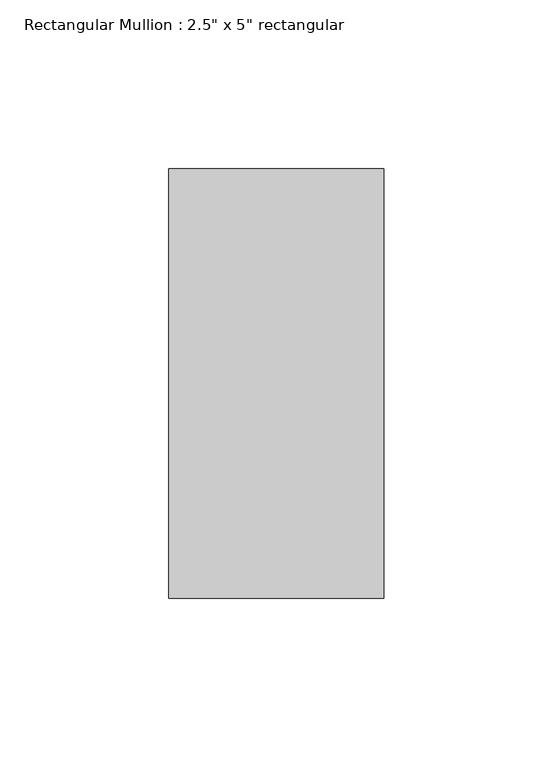
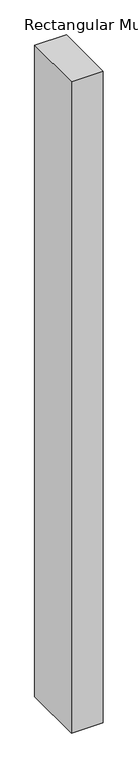
"""IFC4 building model written with IfcOpenShell, lengths in millimetres: member geometry."""

from ifc_helpers import new_model, si_unit, frame, origin, place, context, project, spatial, polyline, outline, extrude, source, transform, mapped, element, save


def member_4dc7c44e(model_context):
    return source(origin(), model_context, "Body", "SweptSolid", [
        extrude(outline(polyline([(31.75, 63.5), (31.75, -63.5), (-31.75, -63.5), (-31.75, 63.5), (31.75, 63.5)])), frame((0.0, 0.0, -1377.95), z_axis=(0.0, 0.0, 1.0), x_axis=(1.0, 0.0, 0.0)), (0.0, 0.0, 1.0), 1377.95),
    ])


if __name__ == "__main__":
    model = new_model("IFC4")
    model_context = context("Model", 3, world=origin())
    ifc_project = project(units=[si_unit("LENGTHUNIT", "METRE", prefix="MILLI")], contexts=[model_context])
    site = spatial("IfcSite", under=ifc_project)
    building = spatial("IfcBuilding", under=site)
    placement = place(None, origin())
    member_shape = member_4dc7c44e(model_context)
    element("IfcMember", 1, ObjectType="Rectangular Mullion : 2.5\" x 5\" rectangular", at=placement, inside=building, context=model_context, shape_type="MappedRepresentation", body=[
        mapped(member_shape, transform((0.0, 0.0, 0.0), x_axis=(1.0, 0.0, 0.0), y_axis=(0.0, 1.0, 0.0), z_axis=(0.0, 0.0, 1.0))),
    ])
    save(model, "model.ifc")

# Revit data of these elements
# Type "Rectangular Mullion : 2.5\" x 5\" rectangular"
#   built-in parameter 1007304 = 0.416667 (stored number, unit not read)
#   built-in parameter 1007301 = 0.104167 (stored number, unit not read)
#   built-in parameter 1007300 = 0.104167 (stored number, unit not read)
# Element 1 (IfcMember, "Rectangular Mullion : 2.5\" x 5\" rectangular")
#   Materials on its faces: "Aluminum"
# Materials
#   "Aluminum": class "Metal", colour RGB 247 247 247, transparency 0, Description = "Aluminum 6061", Cost = 0
